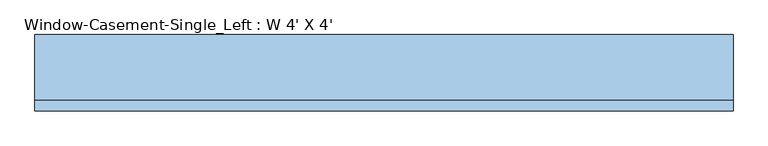
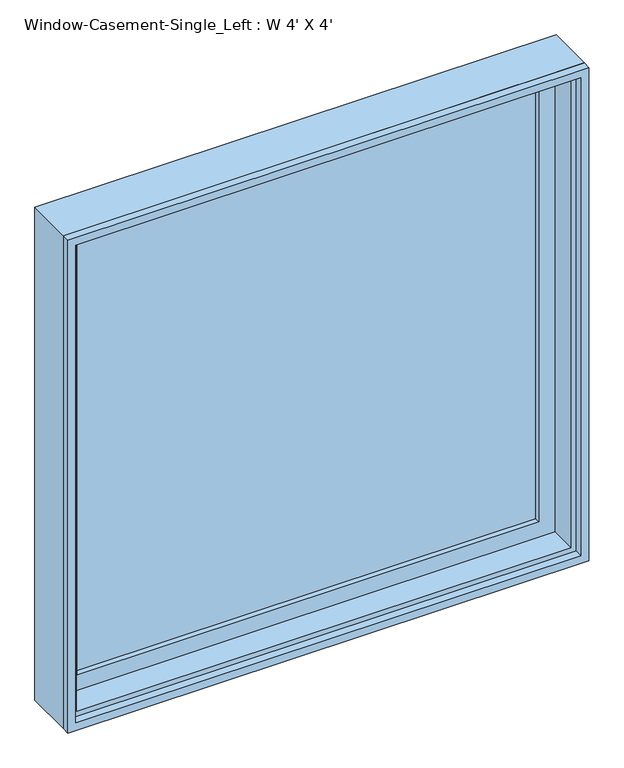
"""IFC4 building model written with IfcOpenShell, lengths in millimetres: window geometry, Window-Casement-Single_Left : W 4' X 4'."""

from ifc_helpers import new_model, si_unit, frame, origin, place, context, project, spatial, polyline, outline, extrude, faceted_brep, source, transform, mapped, element, save


def window_casement_single_left_w_4_x_4_9640c864(model_context):
    return source(origin(), model_context, "Body", "SolidModel", [
        faceted_brep([(577.85, 25.4, 2101.85), (577.85, -38.1, 2101.85), (-577.85, -38.1, 2101.85), (-577.85, 25.4, 2101.85), (596.9, 76.2, 2120.9), (596.9, 25.4, 2120.9), (-596.9, 25.4, 2120.9), (-596.9, 76.2, 2120.9), (609.6, -38.1, 2133.6), (609.6, 76.2, 2133.6), (-609.6, 76.2, 2133.6), (-609.6, -38.1, 2133.6), (-577.85, -38.1, 946.15), (-577.85, 25.4, 946.15), (-596.9, 25.4, 927.1), (-596.9, 76.2, 927.1), (-609.6, 76.2, 914.4), (-609.6, -38.1, 914.4), (577.85, -38.1, 946.15), (577.85, 25.4, 946.15), (596.9, 25.4, 927.1), (596.9, 76.2, 927.1), (609.6, 76.2, 914.4), (609.6, -38.1, 914.4)], [[[0, 1, 2, 3]], [[4, 5, 6, 7]], [[8, 9, 10, 11]], [[3, 2, 12, 13]], [[7, 6, 14, 15]], [[11, 10, 16, 17]], [[13, 12, 18, 19]], [[15, 14, 20, 21]], [[17, 16, 22, 23]], [[11, 17, 23, 8], [1, 18, 12, 2]], [[19, 18, 1, 0]], [[5, 20, 14, 6], [3, 13, 19, 0]], [[21, 20, 5, 4]], [[23, 22, 9, 8]], [[9, 22, 16, 10], [7, 15, 21, 4]]]),
        extrude(outline(polyline([(2133.6, -609.6), (914.4, -609.6), (914.4, 609.6), (2133.6, 609.6), (2133.6, -609.6)]), holes=[polyline([(2114.55, 590.55), (933.45, 590.55), (933.45, -590.55), (2114.55, -590.55), (2114.55, 590.55)])]), frame((0.0, -57.15, 0.0), z_axis=(0.0, 1.0, 0.0), x_axis=(0.0, 0.0, 1.0)), (0.0, 0.0, 1.0), 19.05),
        extrude(outline(polyline([(2120.9, -596.9), (927.1, -596.9), (927.1, 596.9), (2120.9, 596.9), (2120.9, -596.9)]), holes=[polyline([(2063.75, 539.75), (984.25, 539.75), (984.25, -539.75), (2063.75, -539.75), (2063.75, 539.75)])]), frame((0.0, 25.4, 0.0), z_axis=(0.0, 1.0, 0.0), x_axis=(0.0, 0.0, 1.0)), (0.0, 0.0, 1.0), 44.45),
        extrude(outline(polyline([(539.75, 57.15), (539.75, 50.8), (-539.75, 50.8), (-539.75, 57.15), (539.75, 57.15)])), frame((0.0, 0.0, 984.25), z_axis=(0.0, 0.0, 1.0), x_axis=(1.0, 0.0, 0.0)), (0.0, 0.0, 1.0), 1079.5),
        extrude(outline(polyline([(-539.75, 38.1), (-539.75, 44.45), (539.75, 44.45), (539.75, 38.1), (-539.75, 38.1)])), frame((0.0, 0.0, 984.25), z_axis=(0.0, 0.0, 1.0), x_axis=(1.0, 0.0, 0.0)), (0.0, 0.0, 1.0), 1079.5),
    ])


if __name__ == "__main__":
    model = new_model("IFC4")
    model_context = context("Model", 3, world=origin())
    ifc_project = project(units=[si_unit("LENGTHUNIT", "METRE", prefix="MILLI")], contexts=[model_context])
    site = spatial("IfcSite", under=ifc_project)
    building = spatial("IfcBuilding", under=site)
    placement = place(None, origin())
    window_casement_single_left_w_4_x_4_shape = window_casement_single_left_w_4_x_4_9640c864(model_context)
    element("IfcWindow", 1, ObjectType="Window-Casement-Single_Left : W 4' X 4'", at=placement, inside=building, context=model_context, shape_type="MappedRepresentation", body=[
        mapped(window_casement_single_left_w_4_x_4_shape, transform((0.0, 0.0, 0.0), x_axis=(1.0, 0.0, 0.0), y_axis=(0.0, 1.0, 0.0), z_axis=(0.0, 0.0, 1.0))),
    ])
    save(model, "model.ifc")

# Revit data of these elements
# Type "Window-Casement-Single_Left : W 4' X 4'"
#   Type Mark = "19"
#   Fire Rating = "0.5h"
#   Assembly Code = "B2020100"
#   Analytic Construction = "Double glazing - domestic"
#   Window Inset [instance default] = 0' - 0"
#   Wall Thickness [instance default] = 0' - 6"
#   Visual Light Transmittance = 0.81
#   Thermal Resistance (R) = 1.8146 (h·ft²·°F)/BTU
#   Solar Heat Gain Coefficient = 0.76
#   Rough Width = 4' - 0 1/2"
#   Rough Height = 4' - 0 1/2"
#   Interior Wall Closure [instance default] = 0' - 2 1/4"
#   Height = 4' - 0"
#   Heat Transfer Coefficient (U) = 0.5511 BTU/(h·ft²·°F)
#   Frame Extension [instance default] = 0' - 0 1/4"
#   Exterior Wall Closure [instance default] = 0' - 1 1/4"
#   Extension Jamb [instance default] = 0' - 2 1/4"
#   Default Sill Height = 3' - 0"
#   Width = 4' - 0"
#   Muntin Visibility = yes
#   Interior Trim Visibility [instance default] = yes
#   Exterior Trim Visibility [instance default] = yes
#   Extension Jamb Visibility [instance default] = yes
#   Muntin Pattern = Muntin Pattern_2x2 : Muntin Pattern_2x2
#   Interior Trim Material = Wood - Stained
#   Interior Trim = Trim-Window-Interior-Flat : Picture Frame
#   Interior Frame Material = Wood - Stained
#   Glass Panel Material = Glass
#   Exterior Trim Material = Clad - White
#   Exterior Trim = Trim-Window-Exterior-Flat : with Sill
#   Exterior Frame Material = Clad - White
#   Wall Closure = (empty or 0)
# Element 1 (IfcWindow, "Window-Casement-Single_Left : W 4' X 4'")
#   Wall Thickness = 0' - 4 1/2"
#   Extension Jamb = 0' - 0 3/4"
#   Materials on its faces: "Wood - Stained", "Glass", "Clad - White"
# Materials
#   "Wood - Stained": class "Wood", colour RGB 224 178 126, transparency 0, Cost = 0
#   "Glass": class "Glass", colour RGB 0 128 192, transparency 0.75, Description = "Soda Lime Glass", Cost = 0
#   "Clad - White": class "Wood", colour RGB 242 242 238, transparency 0, Cost = 0
